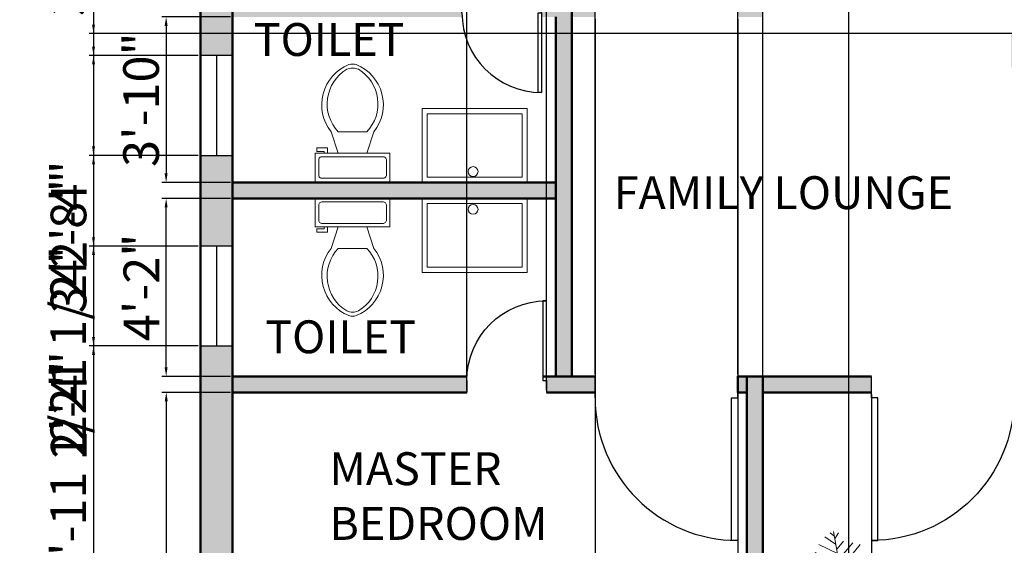
# Model space of a CAD drawing. Units: inches. Extents: x 1344 to 2521, y 3236 to 4924.
# Tile 5 of 14: x 1968 to 2244, y 3472 to 3619. Entities that reach past the tile are written whole.
import ezdxf

# ---------------------------------------------------------------- set-up
doc = ezdxf.new("R2010")
doc.units = ezdxf.units.IN
for name, color, linetype, lineweight in [('A-ANNO-DIMS', 2, 'Continuous', 18), ('A-AREA-IDEN', 3, 'Continuous', 18), ('A-DOOR', 50, 'Continuous', 25), ('A-FLOR-FIXT', 8, 'Continuous', 18), ('A-GLAZ', 150, 'Continuous', 25), ('A-WALL', 31, 'Continuous', 50), ('A-WALL-PATT', 8, 'Continuous', 13), ('L-PLNT', 82, 'Continuous', 13)]:
    doc.layers.add(name, color=color, linetype=linetype, lineweight=lineweight)
doc.styles.get("Standard").update_dxf_attribs({"font": 'arial.ttf'})
doc.dimstyles.new('ISO-25', dxfattribs={"dimtxt": 10, "dimasz": 2.5, "dimexe": 1.25, "dimexo": 0.625, "dimtad": 1, "dimdec": 0, "dimlunit": 4, "dimtxsty": 'Standard', "dimcen": 2.5, "dimadec": 0, "dimazin": 0, "dimtfac": 1, "dimtdec": 0, "dimtmove": 0, "dimatfit": 3, "dimfxl": 1, "dimarcsym": 0})

# ---------------------------------------------------------------- blocks, each defined once
blk = doc.blocks.new('*U2')
for p, q in [((0, 0), (0, -6)), ((40, 0), (40, -6))]:
    blk.add_line(p, q)
blk.add_lwpolyline([(0, 0), (0, 40), (1.75, 40), (1.75, 0)], close=True)
blk.add_arc((0, 0), 40, 0, 90)
blk = doc.blocks.new('*U6')
for p, q in [((9.5, -6), (9.5, -2)), ((-8, -8.5), (-8, -8)), ((-7, -8), (-7, -9.5)), ((-4, -8), (-6, -14)), ((4, -8), (6, -14)), ((-10, -8.5), (-8, -8.5)), ((-10, -9.5), (-10, -8.5)), ((-7, -9.5), (-10, -9.5)), ((4, -14), (-4, -14))]:
    blk.add_line(p, q)
blk.add_lwpolyline([(10.5, -8), (10.5, 0), (-10.5, 0), (-10.5, -8)], close=True)
for points in [[(-9.5, -2), (-9.5, -6)], [(8.5, -1), (-8.5, -1)], [(-8.5, -7), (8.5, -7)]]:
    blk.add_lwpolyline(points)
for centre, radius, start, end in [((-8.62, -1.88), 0.884, 81.8699, 188.1301), ((8.62, -1.88), 0.884, 351.8699, 98.1301), ((-8.62, -6.12), 0.884, 171.8699, 278.1301), ((8.62, -6.12), 0.884, 261.8699, 8.1301), ((3.52, -21.58), 12.17, 141.4691, 247.9714), ((4.2, -21.82), 11.33, 136.3677, 238.9468), ((-3.52, -21.58), 12.17, 292.0284, 38.5307), ((-4.2, -21.82), 11.33, 301.053, 43.6321), ((0, -27.88), 4, 245.7318, 294.2682), ((0, -29), 4, 254.8605, 285.1395)]:
    blk.add_arc(centre, radius, start, end)
blk = doc.blocks.new('*U8')
for p, q in [((-10.186, 53.64), (-13.084, 55.962)), ((0, 0), (-10.5, 57)), ((-9.099, 51.782), (-6.563, 55.962)), ((-7.288, 39.707), (-21.778, 46.673)), ((-8.737, 47.138), (-17.069, 52.711)), ((-7.65, 43.423), (-2.578, 49.46)), ((-5.839, 35.992), (4.667, 48.067)), ((-5.114, 27.632), (10.463, 46.673)), ((-5.114, 28.097), (-24.676, 40.636)), ((-3.665, 19.273), (-27.574, 35.527)), ((-2.941, 16.486), (8.652, 37.85)), ((16.259, 5.805), (23.142, 31.348)), ((22.055, 7.198), (27.489, 32.277)), ((27, 9), (48, 36)), ((27.127, 9.056), (31.112, 35.992)), ((31.836, 30.883), (32.561, 16.486)), ((35.096, 32.741), (37.27, 22.524)), ((38.719, 34.134), (41.979, 28.561)), ((43.791, 29.954), (51.036, 30.883)), ((44.153, 36.456), (45.239, 32.741)), ((-31.5, 4.5), (-52.5, 25.5)), ((-48.585, 21.131), (-49.309, 29.026)), ((-43.513, 28.561), (-42.427, 15.558)), ((-38.442, 26.239), (-34.819, 7.663)), ((-35.544, 28.097), (-24.314, 3.947)), ((-14.533, 2.09), (-30.834, 25.31)), ((-24.314, 23.917), (-2.941, 13.7)), ((-1.129, 6.734), (9.014, 26.704)), ((3.942, 1.625), (11.187, 24.381)), ((10.101, 3.483), (17.708, 26.239)), ((40.53, 25.775), (48.862, 24.846)), ((-47.498, 19.737), (-55.83, 18.344)), ((33.285, 16.486), (48.862, 10.913)), ((36.183, 19.737), (48.137, 17.88)), ((-40.615, 13.7), (-55.105, 10.913)), ((-20.691, 13.7), (-1.129, 4.876)), ((0, 0), (27, 9)), ((29.662, 12.307), (48.137, 6.269)), ((-33.37, 6.269), (-52.207, 5.34)), ((-28.299, 3.483), (-47.86, -5.805)), ((-21.416, 3.018), (-38.079, -8.128)), ((0, 0), (-31.5, 4.5)), ((-15.982, 2.09), (-30.11, -9.521)), ((0, 0), (-22.5, -19.5)), ((-6.563, 1.161), (-21.416, -8.128)), ((0, 0), (18, -22.5)), ((6.478, 1.625), (26.04, -8.592)), ((11.187, 3.483), (30.749, -5.805)), ((18.07, 5.805), (35.096, -3.483)), ((24.229, 7.663), (46.688, 1.625)), ((-6.563, -5.805), (-19.967, -9.985)), ((-4.752, -3.483), (-3.665, -14.629)), ((2.493, -3.019), (-1.491, -20.202)), ((1.769, -2.555), (24.229, -9.521)), ((5.029, -6.27), (2.131, -25.775)), ((-17.431, -15.094), (-42.789, -18.809)), ((-15.257, -12.772), (-30.11, -12.772)), ((-17.069, -15.094), (-12.721, -40.172)), ((-13.446, -11.378), (-8.737, -32.741)), ((-9.461, -8.592), (-6.201, -23.453)), ((9.014, -11.378), (3.58, -35.992)), ((7.565, -9.056), (32.198, -14.629)), ((12.274, -15.094), (36.907, -18.809)), ((-24.314, -21.596), (-42.427, -22.06)), ((-22.5, -19.5), (-37.5, -45)), ((-20.691, -18.345), (-17.793, -44.352)), ((14.085, -16.951), (6.478, -40.172)), ((18.07, -22.524), (8.289, -45.745)), ((16.259, -19.738), (36.183, -22.989)), ((18, -22.5), (27, -52.5)), ((18.433, -22.524), (40.53, -29.026)), ((-28.299, -29.026), (-42.789, -31.348)), ((-26.849, -26.24), (-40.253, -25.775)), ((-25.038, -23.918), (-22.865, -45.281)), ((20.244, -30.419), (15.897, -44.816)), ((19.157, -25.311), (38.719, -33.206)), ((-30.834, -34.135), (-42.427, -35.528)), ((-32.646, -36.921), (-31.921, -44.352)), ((-29.023, -30.884), (-27.936, -43.887)), ((22.78, -37.85), (19.519, -48.532)), ((21.331, -32.741), (39.081, -40.636)), ((22.78, -38.314), (34.372, -44.816)), ((-34.457, -39.708), (-40.978, -42.494)), ((24.591, -45.745), (23.142, -50.854)), ((24.591, -43.423), (30.749, -47.603)), ((26.764, -49.925), (28.213, -50.854))]:
    blk.add_line(p, q)
blk = doc.blocks.new('*D52')
at = {"layer": 'A-ANNO-DIMS', "color": 0, "lineweight": -2, "transparency": 16777216}
for p, q in [((2026.74, 3619.69), (2007.48, 3619.69)), ((2008.73, 3617.19), (2008.73, 3575.82)), ((2026.74, 3573.32), (2007.48, 3573.32))]:
    blk.add_line(p, q, dxfattribs=at)
at = {"layer": 'A-ANNO-DIMS', "color": 0, "lineweight": 100, "transparency": 16777216}
for points in [[(2008.31, 3617.19), (2009.14, 3617.19), (2008.73, 3619.69)], [(2008.31, 3575.82), (2009.14, 3575.82), (2008.73, 3573.32)]]:
    blk.add_solid(points, dxfattribs=at)
at = {"layer": 'Defpoints', "color": 0, "lineweight": 100, "transparency": 16777216}
for p in [(2027.36, 3619.69), (2008.73, 3573.32), (2027.36, 3573.32)]:
    blk.add_point(p, dxfattribs=at)
at = {"layer": 'A-ANNO-DIMS', "color": 0, "transparency": 16777216, "insert": (2002.99, 3596.5), "char_height": 10, "attachment_point": 5, "rotation": 90}
blk.add_mtext('3\'-10"', dxfattribs=at)
blk = doc.blocks.new('*D53')
at = {"layer": 'A-ANNO-DIMS', "color": 0, "lineweight": -2, "transparency": 16777216}
for p, q in [((2026.74, 3568.82), (2007.48, 3568.82)), ((2008.73, 3521.45), (2008.73, 3566.32)), ((2026.74, 3518.95), (2007.48, 3518.95))]:
    blk.add_line(p, q, dxfattribs=at)
at = {"layer": 'A-ANNO-DIMS', "color": 0, "lineweight": 100, "transparency": 16777216}
for points in [[(2008.31, 3566.32), (2009.14, 3566.32), (2008.73, 3568.82)], [(2008.31, 3521.45), (2009.14, 3521.45), (2008.73, 3518.95)]]:
    blk.add_solid(points, dxfattribs=at)
at = {"layer": 'Defpoints', "color": 0, "lineweight": 100, "transparency": 16777216}
for p in [(2008.73, 3568.82), (2027.36, 3568.82), (2027.36, 3518.95)]:
    blk.add_point(p, dxfattribs=at)
at = {"layer": 'A-ANNO-DIMS', "color": 0, "transparency": 16777216, "insert": (2003.08, 3543.88), "char_height": 10, "attachment_point": 5, "rotation": 90}
blk.add_mtext('4\'-2"', dxfattribs=at)
blk = doc.blocks.new('*D54')
at = {"layer": 'A-ANNO-DIMS', "color": 0, "lineweight": -2, "transparency": 16777216}
for p, q in [((2026.74, 3514.45), (2007.52, 3514.45)), ((2008.77, 3511.95), (2008.77, 3358.97)), ((2026.74, 3356.47), (2007.52, 3356.47))]:
    blk.add_line(p, q, dxfattribs=at)
at = {"layer": 'A-ANNO-DIMS', "color": 0, "lineweight": 100, "transparency": 16777216}
for points in [[(2008.35, 3511.95), (2009.18, 3511.95), (2008.77, 3514.45)], [(2008.35, 3358.97), (2009.18, 3358.97), (2008.77, 3356.47)]]:
    blk.add_solid(points, dxfattribs=at)
at = {"layer": 'Defpoints', "color": 0, "lineweight": 100, "transparency": 16777216}
for p in [(2027.36, 3514.45), (2008.77, 3356.47), (2027.36, 3356.47)]:
    blk.add_point(p, dxfattribs=at)
at = {"layer": 'A-ANNO-DIMS', "color": 0, "transparency": 16777216, "insert": (2003.03, 3435.46), "char_height": 10, "attachment_point": 5, "rotation": 90}
blk.add_mtext('13\'-2"', dxfattribs=at)
blk = doc.blocks.new('WASH-BASIN')
for points in [[(29.51, 20.73), (0, 20.73), (0, 0), (29.51, 0)], [(28.05, 19.27), (1.46, 19.27), (1.46, 1.46), (28.05, 1.46)]]:
    blk.add_lwpolyline(points, close=True)
blk.add_circle((14.31, 17.66), 1.38)
blk = doc.blocks.new('*D186')
at = {"layer": 'A-ANNO-DIMS', "color": 0, "lineweight": -2, "transparency": 16777216}
for p, q in [((2017.74, 3763.43), (1987.11, 3763.43)), ((1988.36, 3760.93), (1988.36, 3350.01)), ((2017.74, 3347.51), (1987.11, 3347.51))]:
    blk.add_line(p, q, dxfattribs=at)
at = {"layer": 'A-ANNO-DIMS', "color": 0, "lineweight": 100, "transparency": 16777216}
for points in [[(1987.95, 3760.93), (1988.78, 3760.93), (1988.36, 3763.43)], [(1987.95, 3350.01), (1988.78, 3350.01), (1988.36, 3347.51)]]:
    blk.add_solid(points, dxfattribs=at)
at = {"layer": 'Defpoints', "color": 0, "lineweight": 100, "transparency": 16777216}
for p in [(2018.36, 3763.43), (1988.36, 3347.51), (2018.36, 3347.51)]:
    blk.add_point(p, dxfattribs=at)
at = {"layer": 'A-ANNO-DIMS', "color": 0, "transparency": 16777216, "insert": (1982.63, 3555.47), "char_height": 10, "attachment_point": 5, "rotation": 90}
blk.add_mtext('34\'-8"', dxfattribs=at)
blk = doc.blocks.new('*D196')
at = {"layer": 'A-ANNO-DIMS', "color": 0, "lineweight": -2, "transparency": 16777216}
for p, q in [((2017.74, 3763.43), (1987.11, 3763.43)), ((1988.36, 3760.93), (1988.36, 3611.37)), ((2017.74, 3608.87), (1987.11, 3608.87))]:
    blk.add_line(p, q, dxfattribs=at)
at = {"layer": 'A-ANNO-DIMS', "color": 0, "lineweight": 100, "transparency": 16777216}
for points in [[(1987.95, 3760.93), (1988.78, 3760.93), (1988.36, 3763.43)], [(1987.95, 3611.37), (1988.78, 3611.37), (1988.36, 3608.87)]]:
    blk.add_solid(points, dxfattribs=at)
at = {"layer": 'Defpoints', "color": 0, "lineweight": 100, "transparency": 16777216}
for p in [(2018.36, 3763.43), (1988.36, 3608.87), (2018.36, 3608.87)]:
    blk.add_point(p, dxfattribs=at)
at = {"layer": 'A-ANNO-DIMS', "color": 0, "transparency": 16777216, "insert": (1982.57, 3686.15), "char_height": 10, "attachment_point": 5, "rotation": 90}
blk.add_mtext('12\'-10 1/2"', dxfattribs=at)
blk = doc.blocks.new('*D197')
at = {"layer": 'A-ANNO-DIMS', "color": 0, "lineweight": -2, "transparency": 16777216}
for p, q in [((2017.74, 3608.87), (1987.11, 3608.87)), ((1988.36, 3606.37), (1988.36, 3583.39)), ((2017.74, 3580.89), (1987.11, 3580.89)), ((1988.36, 3580.89), (1988.36, 3550.39))]:
    blk.add_line(p, q, dxfattribs=at)
at = {"layer": 'A-ANNO-DIMS', "color": 0, "lineweight": 100, "transparency": 16777216}
for points in [[(1987.95, 3606.37), (1988.78, 3606.37), (1988.36, 3608.87)], [(1987.95, 3583.39), (1988.78, 3583.39), (1988.36, 3580.89)]]:
    blk.add_solid(points, dxfattribs=at)
at = {"layer": 'Defpoints', "color": 0, "lineweight": 100, "transparency": 16777216}
for p in [(2018.36, 3608.87), (1988.36, 3580.89), (2018.36, 3580.89)]:
    blk.add_point(p, dxfattribs=at)
at = {"layer": 'A-ANNO-DIMS', "color": 0, "transparency": 16777216, "insert": (1982.72, 3564.39), "char_height": 10, "attachment_point": 5, "rotation": 90}
blk.add_mtext('2\'-4"', dxfattribs=at)
blk = doc.blocks.new('*D198')
at = {"layer": 'A-ANNO-DIMS', "color": 0, "lineweight": -2, "transparency": 16777216}
for p, q in [((2017.74, 3580.89), (1987.11, 3580.89)), ((1988.36, 3578.39), (1988.36, 3557.95)), ((2017.74, 3555.45), (1987.11, 3555.45)), ((1988.36, 3555.45), (1988.36, 3501.65))]:
    blk.add_line(p, q, dxfattribs=at)
at = {"layer": 'A-ANNO-DIMS', "color": 0, "lineweight": 100, "transparency": 16777216}
for points in [[(1987.95, 3578.39), (1988.78, 3578.39), (1988.36, 3580.89)], [(1987.95, 3557.95), (1988.78, 3557.95), (1988.36, 3555.45)]]:
    blk.add_solid(points, dxfattribs=at)
at = {"layer": 'Defpoints', "color": 0, "lineweight": 100, "transparency": 16777216}
for p in [(2018.36, 3580.89), (1988.36, 3555.45), (2018.36, 3555.45)]:
    blk.add_point(p, dxfattribs=at)
at = {"layer": 'A-ANNO-DIMS', "color": 0, "transparency": 16777216, "insert": (1982.57, 3527.3), "char_height": 10, "attachment_point": 5, "rotation": 90}
blk.add_mtext('2\'-1 1/2"', dxfattribs=at)
blk = doc.blocks.new('*D199')
at = {"layer": 'A-ANNO-DIMS', "color": 0, "lineweight": -2, "transparency": 16777216}
for p, q in [((2017.74, 3555.45), (1987.11, 3555.45)), ((1988.36, 3552.95), (1988.36, 3529.97)), ((2017.74, 3527.47), (1987.11, 3527.47)), ((1988.36, 3527.47), (1988.36, 3496.97))]:
    blk.add_line(p, q, dxfattribs=at)
at = {"layer": 'A-ANNO-DIMS', "color": 0, "lineweight": 100, "transparency": 16777216}
for points in [[(1987.95, 3552.95), (1988.78, 3552.95), (1988.36, 3555.45)], [(1987.95, 3529.97), (1988.78, 3529.97), (1988.36, 3527.47)]]:
    blk.add_solid(points, dxfattribs=at)
at = {"layer": 'Defpoints', "color": 0, "lineweight": 100, "transparency": 16777216}
for p in [(2018.36, 3555.45), (1988.36, 3527.47), (2018.36, 3527.47)]:
    blk.add_point(p, dxfattribs=at)
at = {"layer": 'A-ANNO-DIMS', "color": 0, "transparency": 16777216, "insert": (1982.72, 3510.97), "char_height": 10, "attachment_point": 5, "rotation": 90}
blk.add_mtext('2\'-4"', dxfattribs=at)
blk = doc.blocks.new('*D200')
at = {"layer": 'A-ANNO-DIMS', "color": 0, "lineweight": -2, "transparency": 16777216}
for p, q in [((2017.74, 3527.47), (1987.11, 3527.47)), ((1988.36, 3524.97), (1988.36, 3458.32)), ((2017.74, 3455.82), (1987.11, 3455.82))]:
    blk.add_line(p, q, dxfattribs=at)
at = {"layer": 'A-ANNO-DIMS', "color": 0, "lineweight": 100, "transparency": 16777216}
for points in [[(1987.95, 3524.97), (1988.78, 3524.97), (1988.36, 3527.47)], [(1987.95, 3458.32), (1988.78, 3458.32), (1988.36, 3455.82)]]:
    blk.add_solid(points, dxfattribs=at)
at = {"layer": 'Defpoints', "color": 0, "lineweight": 100, "transparency": 16777216}
for p in [(2018.36, 3527.47), (1988.36, 3455.82), (2018.36, 3455.82)]:
    blk.add_point(p, dxfattribs=at)
at = {"layer": 'A-ANNO-DIMS', "color": 0, "transparency": 16777216, "insert": (1982.57, 3491.65), "char_height": 10, "attachment_point": 5, "rotation": 90}
blk.add_mtext('5\'-11 1/2"', dxfattribs=at)
blk = doc.blocks.new('*D209')
at = {"layer": 'A-ANNO-DIMS', "color": 0, "lineweight": -2, "transparency": 16777216}
for p, q in [((2129.02, 3619.06), (2129.02, 3316.22)), ((2169.02, 3619.06), (2169.02, 3316.22)), ((2131.52, 3317.47), (2166.52, 3317.47))]:
    blk.add_line(p, q, dxfattribs=at)
at = {"layer": 'A-ANNO-DIMS', "color": 0, "lineweight": 100, "transparency": 16777216}
for points in [[(2131.52, 3317.89), (2131.52, 3317.06), (2129.02, 3317.47)], [(2166.52, 3317.89), (2166.52, 3317.06), (2169.02, 3317.47)]]:
    blk.add_solid(points, dxfattribs=at)
at = {"layer": 'Defpoints', "color": 0, "lineweight": 100, "transparency": 16777216}
for p in [(2129.02, 3619.69), (2169.02, 3619.69), (2169.02, 3317.47)]:
    blk.add_point(p, dxfattribs=at)
at = {"layer": 'A-ANNO-DIMS', "color": 0, "transparency": 16777216, "insert": (2149.02, 3323.21), "char_height": 10, "attachment_point": 5}
blk.add_mtext('3\'-4"', dxfattribs=at)
blk = doc.blocks.new('*D210')
at = {"layer": 'A-ANNO-DIMS', "color": 0, "lineweight": -2, "transparency": 16777216}
for p, q in [((2093.06, 3515.07), (2093.06, 3794.68)), ((2115.39, 3515.07), (2115.39, 3794.68)), ((2095.56, 3793.43), (2112.89, 3793.43)), ((2115.39, 3793.43), (2175.85, 3793.43))]:
    blk.add_line(p, q, dxfattribs=at)
at = {"layer": 'A-ANNO-DIMS', "color": 0, "lineweight": 100, "transparency": 16777216}
for points in [[(2095.56, 3793.85), (2095.56, 3793.02), (2093.06, 3793.43)], [(2112.89, 3793.85), (2112.89, 3793.02), (2115.39, 3793.43)]]:
    blk.add_solid(points, dxfattribs=at)
at = {"layer": 'Defpoints', "color": 0, "lineweight": 100, "transparency": 16777216}
for p in [(2115.39, 3793.43), (2093.06, 3514.45), (2115.39, 3514.45)]:
    blk.add_point(p, dxfattribs=at)
at = {"layer": 'A-ANNO-DIMS', "color": 0, "transparency": 16777216, "insert": (2146.87, 3799.23), "char_height": 10, "attachment_point": 5}
blk.add_mtext('1\'-10 1/2"', dxfattribs=at)
blk = doc.blocks.new('*D211')
at = {"layer": 'A-ANNO-DIMS', "color": 0, "lineweight": -2, "transparency": 16777216}
for p, q in [((2129.02, 3519.57), (2129.02, 3794.68)), ((2169.02, 3519.57), (2169.02, 3794.68)), ((2131.52, 3793.43), (2166.52, 3793.43))]:
    blk.add_line(p, q, dxfattribs=at)
at = {"layer": 'A-ANNO-DIMS', "color": 0, "lineweight": 100, "transparency": 16777216}
for points in [[(2131.52, 3793.85), (2131.52, 3793.02), (2129.02, 3793.43)], [(2166.52, 3793.85), (2166.52, 3793.02), (2169.02, 3793.43)]]:
    blk.add_solid(points, dxfattribs=at)
at = {"layer": 'Defpoints', "color": 0, "lineweight": 100, "transparency": 16777216}
for p in [(2169.02, 3793.43), (2129.02, 3518.95), (2169.02, 3518.95)]:
    blk.add_point(p, dxfattribs=at)
at = {"layer": 'A-ANNO-DIMS', "color": 0, "transparency": 16777216, "insert": (2149.02, 3799.17), "char_height": 10, "attachment_point": 5}
blk.add_mtext('3\'-4"', dxfattribs=at)
blk = doc.blocks.new('*D214')
at = {"layer": 'A-ANNO-DIMS', "color": 0, "lineweight": -2, "transparency": 16777216}
for p, q in [((2249.66, 3655.04), (1987.11, 3655.04)), ((1988.36, 3652.54), (1988.36, 3617.54)), ((2249.66, 3615.04), (1987.11, 3615.04))]:
    blk.add_line(p, q, dxfattribs=at)
at = {"layer": 'A-ANNO-DIMS', "color": 0, "lineweight": 100, "transparency": 16777216}
for points in [[(1987.95, 3652.54), (1988.78, 3652.54), (1988.36, 3655.04)], [(1987.95, 3617.54), (1988.78, 3617.54), (1988.36, 3615.04)]]:
    blk.add_solid(points, dxfattribs=at)
at = {"layer": 'Defpoints', "color": 0, "lineweight": 100, "transparency": 16777216}
for p in [(2250.29, 3655.04), (1988.36, 3615.04), (2250.29, 3615.04)]:
    blk.add_point(p, dxfattribs=at)
at = {"layer": 'A-ANNO-DIMS', "color": 0, "transparency": 16777216, "insert": (1982.63, 3635.04), "char_height": 10, "attachment_point": 5, "rotation": 90}
blk.add_mtext('3\'-4"', dxfattribs=at)
blk = doc.blocks.new('*D215')
at = {"layer": 'A-ANNO-DIMS', "color": 0, "lineweight": -2, "transparency": 16777216}
for p, q in [((2206.56, 3513.82), (2206.56, 3316.22)), ((2246.56, 3513.82), (2246.56, 3316.22)), ((2209.06, 3317.47), (2244.06, 3317.47))]:
    blk.add_line(p, q, dxfattribs=at)
at = {"layer": 'A-ANNO-DIMS', "color": 0, "lineweight": 100, "transparency": 16777216}
for points in [[(2209.06, 3317.89), (2209.06, 3317.06), (2206.56, 3317.47)], [(2244.06, 3317.89), (2244.06, 3317.06), (2246.56, 3317.47)]]:
    blk.add_solid(points, dxfattribs=at)
at = {"layer": 'Defpoints', "color": 0, "lineweight": 100, "transparency": 16777216}
for p in [(2206.56, 3514.45), (2246.56, 3514.45), (2246.56, 3317.47)]:
    blk.add_point(p, dxfattribs=at)
at = {"layer": 'A-ANNO-DIMS', "color": 0, "transparency": 16777216, "insert": (2226.56, 3323.21), "char_height": 10, "attachment_point": 5}
blk.add_mtext('3\'-4"', dxfattribs=at)
blk = doc.blocks.new('*D216')
at = {"layer": 'A-ANNO-DIMS', "color": 0, "lineweight": -2, "transparency": 16777216}
for p, q in [((2176.1, 3403.64), (2176.1, 3794.68)), ((2200.2, 3403.64), (2200.2, 3794.68)), ((2178.6, 3793.43), (2197.7, 3793.43)), ((2200.2, 3793.43), (2230.7, 3793.43))]:
    blk.add_line(p, q, dxfattribs=at)
at = {"layer": 'A-ANNO-DIMS', "color": 0, "lineweight": 100, "transparency": 16777216}
for points in [[(2178.6, 3793.85), (2178.6, 3793.02), (2176.1, 3793.43)], [(2197.7, 3793.85), (2197.7, 3793.02), (2200.2, 3793.43)]]:
    blk.add_solid(points, dxfattribs=at)
at = {"layer": 'Defpoints', "color": 0, "lineweight": 100, "transparency": 16777216}
for p in [(2200.2, 3793.43), (2176.1, 3403.01), (2200.2, 3403.01)]:
    blk.add_point(p, dxfattribs=at)
at = {"layer": 'A-ANNO-DIMS', "color": 0, "transparency": 16777216, "insert": (2216.7, 3799.16), "char_height": 10, "attachment_point": 5}
blk.add_mtext('2\'-0"', dxfattribs=at)
blk = doc.blocks.new('*D217')
at = {"layer": 'A-ANNO-DIMS', "color": 0, "lineweight": -2, "transparency": 16777216}
for p, q in [((2200.2, 3403.64), (2200.2, 3794.68)), ((2345.46, 3403.64), (2345.46, 3794.68)), ((2202.7, 3793.43), (2342.96, 3793.43))]:
    blk.add_line(p, q, dxfattribs=at)
at = {"layer": 'A-ANNO-DIMS', "color": 0, "lineweight": 100, "transparency": 16777216}
for points in [[(2202.7, 3793.85), (2202.7, 3793.02), (2200.2, 3793.43)], [(2342.96, 3793.85), (2342.96, 3793.02), (2345.46, 3793.43)]]:
    blk.add_solid(points, dxfattribs=at)
at = {"layer": 'Defpoints', "color": 0, "lineweight": 100, "transparency": 16777216}
for p in [(2345.46, 3793.43), (2200.2, 3403.01), (2345.46, 3403.01)]:
    blk.add_point(p, dxfattribs=at)
at = {"layer": 'A-ANNO-DIMS', "color": 0, "transparency": 16777216, "insert": (2272.83, 3799.23), "char_height": 10, "attachment_point": 5}
blk.add_mtext('12\'-1 1/2"', dxfattribs=at)

msp = doc.modelspace()

# ---------------------------------------------------------------- hatches: boundary and pattern name
at = {"layer": 'A-WALL-PATT'}
h = msp.add_hatch(color=256, dxfattribs=at)
h.dxf.hatch_style = 1
h.paths.add_polyline_path([(2193.45, 3763.43), (2126.57, 3763.43), (2126.57, 3754.43), (2193.45, 3754.43)])
h.paths.add_polyline_path([(2057.65, 3763.43), (2018.36, 3763.43), (2018.36, 3608.87), (2027.36, 3608.87), (2027.36, 3754.43), (2057.65, 3754.43)])
h.paths.add_polyline_path([(2266.48, 3763.43), (2226.56, 3763.43), (2226.56, 3754.43), (2266.48, 3754.43)])
h.paths.add_polyline_path([(2378.36, 3763.43), (2335.41, 3763.43), (2335.41, 3754.43), (2369.36, 3754.43), (2369.36, 3594.28), (2378.36, 3594.28)])
h.paths.add_polyline_path([(2369.36, 3610.02), (2250.29, 3610.02), (2250.29, 3605.52), (2369.36, 3605.52)])
h.paths.add_polyline_path([(2250.29, 3610.02), (2245.79, 3610.02), (2245.79, 3605.52), (2250.29, 3605.52)])
h.paths.add_polyline_path([(2250.29, 3754.43), (2245.79, 3754.43), (2245.79, 3655.04), (2250.29, 3655.04)])
h.paths.add_polyline_path([(2176.1, 3754.43), (2171.6, 3754.43), (2171.6, 3624.19), (2171.35, 3624.19), (2169.02, 3624.19), (2169.02, 3619.69), (2176.1, 3619.69)])
h.paths.add_polyline_path([(2129.02, 3624.19), (2122.52, 3624.19), (2122.52, 3619.69), (2129.02, 3619.69)])
h.paths.add_polyline_path([(2091.69, 3624.19), (2027.36, 3624.19), (2027.36, 3619.69), (2091.72, 3619.69, -0.012876), (2091.69, 3620.84)])
h.paths.add_polyline_path([(2250.29, 3615.04), (2245.79, 3615.04), (2245.79, 3610.02), (2250.29, 3610.02)])
h.paths.add_polyline_path([(2027.36, 3580.89), (2018.36, 3580.89), (2018.36, 3555.45), (2027.36, 3555.45)])
h.paths.add_polyline_path([(2027.36, 3527.47), (2018.36, 3527.47), (2018.36, 3455.82), (2027.36, 3455.82)])
h.paths.add_polyline_path([(2093.06, 3517.8, -0.012876), (2093.09, 3518.95), (2027.36, 3518.95), (2027.36, 3514.45), (2093.06, 3514.45)])
h.paths.add_polyline_path([(2118.02, 3573.32), (2110.02, 3573.32), (2110.02, 3573.28), (2080.51, 3573.28), (2027.36, 3573.32), (2027.36, 3568.82), (2118.02, 3568.82)])
h.paths.add_polyline_path([(2122.52, 3624.19), (2114.02, 3624.19), (2114.02, 3620.84), (2114.02, 3619.69), (2118.02, 3619.69), (2118.02, 3518.95), (2122.52, 3518.95)])
h.paths.add_polyline_path([(2129.02, 3518.95), (2115.39, 3518.95), (2115.39, 3517.8), (2115.39, 3514.45), (2129.02, 3514.45)])
h.paths.add_polyline_path([(2027.36, 3386.9), (2018.36, 3386.9), (2018.36, 3347.51), (2056.7, 3347.51), (2056.7, 3356.47), (2027.36, 3356.47)])
h.paths.add_polyline_path([(2187.76, 3356.47), (2168.81, 3356.47), (2149.67, 3356.47), (2125.62, 3356.47), (2125.62, 3347.51), (2176.1, 3347.51), (2187.76, 3347.51)])
h.paths.add_polyline_path([(2378.36, 3525.36), (2369.36, 3525.36), (2369.36, 3497.27), (2369.36, 3412.01), (2369.57, 3412.01), (2369.57, 3403.01), (2369.36, 3356.51), (2369.36, 3347.51), (2378.36, 3347.51)])
h.paths.add_polyline_path([(2369.36, 3412.01), (2345.46, 3412.01), (2345.46, 3403.01), (2369.36, 3403.01)])
h.paths.add_polyline_path([(2206.56, 3518.95), (2176.1, 3518.95), (2176.1, 3514.45), (2206.56, 3514.45)])
h.paths.add_polyline_path([(2130.92, 3560.64), (2239.92, 3560.64), (2239.92, 3579.62), (2130.92, 3579.62)], flags=9)
h.paths.add_polyline_path([(2271.24, 3730.09), (2345.91, 3730.09), (2345.91, 3749.07), (2271.24, 3749.07)], flags=9)
h.paths.add_polyline_path([(2051.28, 3467.76), (2122.39, 3467.76), (2122.39, 3502.26), (2051.28, 3502.26)], flags=9)
h.paths.add_polyline_path([(2033.92, 3520.24), (2083.56, 3520.24), (2083.56, 3539.22), (2033.92, 3539.22)], flags=9)
h.paths.add_polyline_path([(2030.69, 3603.57), (2080.34, 3603.57), (2080.34, 3622.55), (2030.69, 3622.55)], flags=9)
h.paths.add_polyline_path([(2175.78, 3699.42), (2225.43, 3699.42), (2225.43, 3718.41), (2175.78, 3718.41)], flags=9)
h.paths.add_polyline_path([(2051.88, 3718.72), (2122.99, 3718.72), (2122.99, 3753.22), (2051.88, 3753.22)], flags=9)
h = msp.add_hatch(color=256, dxfattribs=at)
h.dxf.hatch_style = 1
h.paths.add_polyline_path([(2200.2, 3412.01), (2176.1, 3412.01), (2176.1, 3403.01), (2200.2, 3403.01)])
h.paths.add_polyline_path([(2369.36, 3518.95), (2246.56, 3518.95), (2246.56, 3514.45), (2369.36, 3514.45)])
h.paths.add_polyline_path([(2130.92, 3560.64), (2239.92, 3560.64), (2239.92, 3579.62), (2130.92, 3579.62)], flags=9)
h.paths.add_polyline_path([(2271.24, 3730.09), (2345.91, 3730.09), (2345.91, 3749.07), (2271.24, 3749.07)], flags=9)
h.paths.add_polyline_path([(2051.28, 3467.76), (2122.39, 3467.76), (2122.39, 3502.26), (2051.28, 3502.26)], flags=9)
h.paths.add_polyline_path([(2033.92, 3520.24), (2083.56, 3520.24), (2083.56, 3539.22), (2033.92, 3539.22)], flags=9)
h.paths.add_polyline_path([(2030.69, 3603.57), (2080.34, 3603.57), (2080.34, 3622.55), (2030.69, 3622.55)], flags=9)
h.paths.add_polyline_path([(2175.78, 3699.42), (2225.43, 3699.42), (2225.43, 3718.41), (2175.78, 3718.41)], flags=9)
h.paths.add_polyline_path([(2051.88, 3718.72), (2122.99, 3718.72), (2122.99, 3753.22), (2051.88, 3753.22)], flags=9)
h = msp.add_hatch(color=256, dxfattribs=at)
h.dxf.hatch_style = 1
h.paths.add_polyline_path([(2176.1, 3518.95), (2171.6, 3518.95), (2171.6, 3514.45), (2171.6, 3356.47), (2176.1, 3356.47)])
h.paths.add_polyline_path([(2171.6, 3518.95), (2169.02, 3518.95), (2169.02, 3514.45), (2171.6, 3514.45)])

# ---------------------------------------------------------------- linework, layer by layer
at = {"layer": 'A-GLAZ'}
for p, q in [((2022.86, 3608.87), (2022.86, 3580.89)), ((2022.86, 3555.45), (2022.86, 3527.47))]:
    msp.add_line(p, q, dxfattribs=at)
for points in [[(2027.36, 3608.87), (2018.36, 3608.87), (2018.36, 3580.89), (2027.36, 3580.89)], [(2027.36, 3555.45), (2018.36, 3555.45), (2018.36, 3527.47), (2027.36, 3527.47)]]:
    msp.add_lwpolyline(points, close=True, dxfattribs=at)
at = {"layer": 'A-WALL'}
for p, q in [((2122.52, 3624.19), (2122.52, 3518.95)), ((2118.02, 3619.69), (2118.02, 3518.95)), ((2027.36, 3573.32), (2118.02, 3573.32)), ((2027.36, 3568.82), (2118.02, 3568.82)), ((2027.36, 3518.95), (2093.09, 3518.95)), ((2114.41, 3518.95), (2129.02, 3518.95)), ((2169.02, 3518.95), (2171.6, 3518.95)), ((2176.1, 3518.95), (2169.02, 3518.95)), ((2174.53, 3518.95), (2206.56, 3518.95)), ((2176.1, 3514.45), (2176.1, 3518.95)), ((2027.36, 3514.45), (2093.06, 3514.45)), ((2115.39, 3514.45), (2129.02, 3514.45)), ((2169.02, 3514.45), (2171.6, 3514.45)), ((2171.6, 3514.45), (2171.6, 3356.47)), ((2176.1, 3514.45), (2176.1, 3356.47)), ((2176.1, 3514.45), (2206.56, 3514.45))]:
    msp.add_line(p, q, dxfattribs=at)
for points in [[(2378.36, 3347.51), (2378.36, 3763.43), (2018.36, 3763.43), (2018.36, 3347.51)], [(2369.36, 3356.51), (2369.36, 3754.43), (2027.36, 3754.43), (2027.36, 3356.47)]]:
    msp.add_lwpolyline(points, dxfattribs=at)
for points in [[(2171.6, 3514.45), (2169.02, 3514.45), (2169.02, 3518.95), (2171.6, 3518.95)], [(2171.6, 3356.47), (2176.1, 3356.47), (2176.1, 3518.95), (2171.6, 3518.95)]]:
    msp.add_lwpolyline(points, close=True, dxfattribs=at)

# ---------------------------------------------------------------- block references
at = {"layer": 'A-DOOR', "xscale": 0.5583757449765673, "yscale": 0.5583757449765673, "zscale": 0.5583757449765673, "rotation": 180}
msp.add_blockref('*U2', (2114.02, 3620.84), dxfattribs=at)
at = {"layer": 'A-DOOR', "xscale": -0.5583757449765673, "yscale": 0.5583757449765673, "zscale": 0.5583757449765673}
msp.add_blockref('*U2', (2115.39, 3517.8), dxfattribs=at)
at = {"layer": 'A-DOOR', "rotation": 180}
msp.add_blockref('*U2', (2169.02, 3512.95), dxfattribs=at)
at = {"layer": 'A-DOOR', "xscale": -1, "rotation": 180}
msp.add_blockref('*U2', (2206.56, 3512.95), dxfattribs=at)
at = {"layer": 'A-FLOR-FIXT', "xscale": -1, "rotation": 180}
msp.add_blockref('*U6', (2061.01, 3573.49), dxfattribs=at)
at = {"layer": 'A-FLOR-FIXT', "extrusion": (0, 0, -1), "zscale": -1, "rotation": 180}
msp.add_blockref('WASH-BASIN', (-2080.51, 3594.01), dxfattribs=at)
at = {"layer": 'A-FLOR-FIXT'}
for name, p in [('*U6', (2061.01, 3568.82)), ('WASH-BASIN', (2080.51, 3548.09))]:
    msp.add_blockref(name, p, dxfattribs=at)
at = {"layer": 'L-PLNT', "xscale": 0.3591539065448135, "yscale": 0.3591539065448135, "zscale": 0.3591539065448135}
msp.add_blockref('*U8', (2199.64, 3455.01), dxfattribs=at)

# ---------------------------------------------------------------- texts
at = {"layer": 'A-AREA-IDEN', "char_height": 9.211, "attachment_point": 1}
for s, insert in [('TOILET', (2033.3, 3617.97)), ('FAMILY LOUNGE', (2134.28, 3575.04)), ('TOILET', (2036.52, 3534.64)), ('MASTER BEDROOM', (2054.54, 3497.67))]:
    msp.add_mtext_dynamic_manual_height_columns(s, width=108.7809, gutter_width=46.06, heights=[0], dxfattribs=dict(at, insert=insert))

# ---------------------------------------------------------------- dimensions: what is measured, and where the dimension line sits
at = {"layer": 'A-ANNO-DIMS'}
for base, p1, p2, picture, middle in [((2115.39, 3793.43), (2093.06, 3514.45), (2115.39, 3514.45), '*D210', (2146.87, 3799.23)), ((2345.46, 3793.43), (2200.2, 3403.01), (2345.46, 3403.01), '*D217', (2272.83, 3799.23)), ((2169.02, 3793.43), (2129.02, 3518.95), (2169.02, 3518.95), '*D211', (2149.02, 3799.17)), ((2200.2, 3793.43), (2176.1, 3403.01), (2200.2, 3403.01), '*D216', (2216.7, 3799.16)), ((2169.02, 3317.47), (2129.02, 3619.69), (2169.02, 3619.69), '*D209', (2149.02, 3323.21)), ((2246.56, 3317.47), (2206.56, 3514.45), (2246.56, 3514.45), '*D215', (2226.56, 3323.21))]:
    dim = msp.add_linear_dim(base=base, p1=p1, p2=p2, dimstyle='ISO-25', override={"dimdec": 1, "dimlfac": 1, "dimrnd": 0, "dimzin": 1, "dimdsep": 46, "dimlunit": 4, "dimfrac": 2}, dxfattribs=at)
    dim.commit()
    dim.dimension.update_dxf_attribs({"geometry": picture, "text_midpoint": middle})
for base, p1, p2, override, picture, middle in [((1988.36, 3608.87), (2018.36, 3763.43), (2018.36, 3608.87), {"dimdec": 1, "dimlfac": 1, "dimrnd": 0, "dimzin": 1, "dimdsep": 46, "dimlunit": 4, "dimfrac": 2}, '*D196', (1982.57, 3686.15)), ((1988.36, 3347.51), (2018.36, 3763.43), (2018.36, 3347.51), {"dimdec": 1, "dimlfac": 1, "dimrnd": 0, "dimzin": 1, "dimdsep": 46, "dimlunit": 4, "dimfrac": 2}, '*D186', (1982.63, 3555.47)), ((1988.36, 3615.04), (2250.29, 3655.04), (2250.29, 3615.04), {"dimdec": 1, "dimlfac": 1, "dimrnd": 0, "dimzin": 1, "dimdsep": 46, "dimlunit": 4, "dimfrac": 2}, '*D214', (1982.63, 3635.04)), ((2008.73, 3573.32), (2027.36, 3619.69), (2027.36, 3573.32), {"dimclrd": 0, "dimclre": 0, "dimclrt": 0}, '*D52', (2002.99, 3596.5)), ((1988.36, 3580.89), (2018.36, 3608.87), (2018.36, 3580.89), {"dimdec": 1, "dimlfac": 1, "dimrnd": 0, "dimzin": 1, "dimdsep": 46, "dimlunit": 4, "dimfrac": 2}, '*D197', (1982.72, 3564.39)), ((1988.36, 3555.45), (2018.36, 3580.89), (2018.36, 3555.45), {"dimdec": 1, "dimlfac": 1, "dimrnd": 0, "dimzin": 1, "dimdsep": 46, "dimlunit": 4, "dimfrac": 2}, '*D198', (1982.57, 3527.3)), ((2008.73, 3568.82), (2027.36, 3518.95), (2027.36, 3568.82), {"dimclrd": 0, "dimclre": 0, "dimclrt": 0}, '*D53', (2003.08, 3543.88)), ((1988.36, 3527.47), (2018.36, 3555.45), (2018.36, 3527.47), {"dimdec": 1, "dimlfac": 1, "dimrnd": 0, "dimzin": 1, "dimdsep": 46, "dimlunit": 4, "dimfrac": 2}, '*D199', (1982.72, 3510.97)), ((1988.3631, 3455.8226), (2018.3631, 3527.4742), (2018.3631, 3455.8226), {"dimdec": 1, "dimlfac": 1, "dimrnd": 0, "dimzin": 1, "dimdsep": 46, "dimlunit": 4, "dimfrac": 2}, '*D200', (1982.5676, 3491.6484)), ((2008.77, 3356.47), (2027.36, 3514.45), (2027.36, 3356.47), {"dimclrd": 0, "dimclre": 0, "dimclrt": 0}, '*D54', (2003.03, 3435.46))]:
    dim = msp.add_linear_dim(base=base, p1=p1, p2=p2, angle=90, dimstyle='ISO-25', override=override, dxfattribs=at)
    dim.commit()
    dim.dimension.update_dxf_attribs({"geometry": picture, "text_midpoint": middle})

doc.saveas('drawing.dxf')
